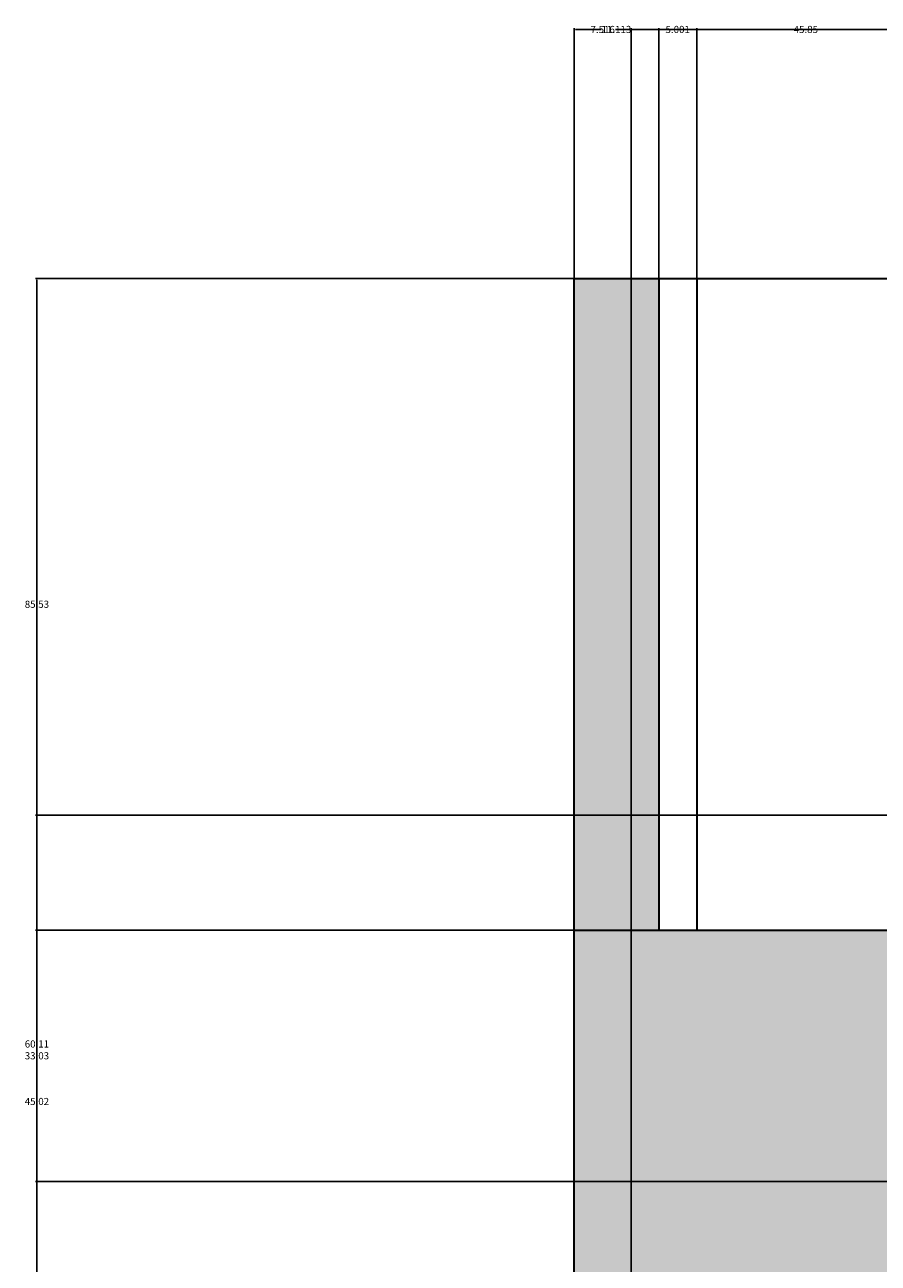
# Model space of a CAD drawing. Units: inches. Extents: x -5 to 714, y 84 to 644.
# Tile 9 of 20: x -4 to 108, y 481 to 644. Entities that reach past the tile are written whole.
import ezdxf

# ---------------------------------------------------------------- set-up
doc = ezdxf.new("R2010")
doc.units = ezdxf.units.IN
doc.header["$MEASUREMENT"] = 0
for name, color, linetype, lineweight in [('A-ANNO-DIMS', 2, 'Continuous', 18), ('A-ELEV', 7, 'Continuous', 35), ('A-ELEV-PATT', 8, 'Continuous', 13)]:
    doc.layers.add(name, color=color, linetype=linetype, lineweight=lineweight)
doc.styles.get("Standard").update_dxf_attribs({"font": 'arial.ttf'})
doc.dimstyles.get("Standard").update_dxf_attribs({"dimtxt": 0.9375, "dimasz": 0.18, "dimexe": 0.18, "dimexo": 0.0625, "dimgap": 0.09, "dimtad": 0, "dimtih": 1, "dimtoh": 1, "dimdec": 4, "dimzin": 0, "dimdsep": 46, "dimlunit": 4, "dimtxsty": 'Standard', "dimcen": 0.09, "dimadec": 0, "dimazin": 0, "dimtfac": 1, "dimtdec": 4, "dimtofl": 0, "dimtmove": 0, "dimatfit": 3, "dimfxl": 1, "dimtolj": 1, "dimtzin": 0, "dimarcsym": 0})

# ---------------------------------------------------------------- blocks, each defined once
blk = doc.blocks.new('*D2')
at = {"layer": 'A-ANNO-DIMS', "color": 0, "lineweight": -2, "transparency": 16777216}
for p, q in [((67.93, 610.73), (-2.74, 610.73)), ((-2.56, 610.55), (-2.56, 364.53)), ((-2.56, 117.37), (-2.56, 363.39)), ((30.08, 117.19), (-2.74, 117.19))]:
    blk.add_line(p, q, dxfattribs=at)
at = {"layer": 'A-ANNO-DIMS', "color": 0, "transparency": 16777216}
for points in [[(-2.59, 610.55), (-2.53, 610.55), (-2.56, 610.73)], [(-2.59, 117.37), (-2.53, 117.37), (-2.56, 117.19)]]:
    blk.add_solid(points, dxfattribs=at)
at = {"layer": 'Defpoints', "color": 0, "transparency": 16777216}
for p in [(-2.56, 610.73), (67.99, 610.73), (30.14, 117.19)]:
    blk.add_point(p, dxfattribs=at)
at = {"layer": 'A-ANNO-DIMS', "color": 0, "transparency": 16777216, "insert": (-2.56, 363.96), "char_height": 0.938, "attachment_point": 5}
blk.add_mtext('\\A1;493.5', dxfattribs=at)
blk = doc.blocks.new('*D6')
at = {"layer": 'A-ANNO-DIMS', "color": 0, "lineweight": -2, "transparency": 16777216}
for p, q in [((67.93, 525.19), (-2.74, 525.19)), ((-2.56, 525.01), (-2.56, 435.76)), ((-2.56, 345.37), (-2.56, 434.62)), ((67.93, 345.19), (-2.74, 345.19))]:
    blk.add_line(p, q, dxfattribs=at)
at = {"layer": 'A-ANNO-DIMS', "color": 0, "transparency": 16777216}
for points in [[(-2.59, 525.01), (-2.53, 525.01), (-2.56, 525.19)], [(-2.59, 345.37), (-2.53, 345.37), (-2.56, 345.19)]]:
    blk.add_solid(points, dxfattribs=at)
at = {"layer": 'Defpoints', "color": 0, "transparency": 16777216}
for p in [(-2.56, 525.19), (67.99, 525.19), (67.99, 345.19)]:
    blk.add_point(p, dxfattribs=at)
at = {"layer": 'A-ANNO-DIMS', "color": 0, "transparency": 16777216, "insert": (-2.56, 435.19), "char_height": 0.938, "attachment_point": 5}
blk.add_mtext('\\A1;180', dxfattribs=at)
blk = doc.blocks.new('*D7')
at = {"layer": 'A-ANNO-DIMS', "color": 0, "lineweight": -2, "transparency": 16777216}
for p, q in [((67.93, 610.73), (-2.74, 610.73)), ((-2.56, 610.55), (-2.56, 568.53)), ((-2.56, 525.37), (-2.56, 567.39)), ((67.93, 525.19), (-2.74, 525.19))]:
    blk.add_line(p, q, dxfattribs=at)
at = {"layer": 'A-ANNO-DIMS', "color": 0, "transparency": 16777216}
for points in [[(-2.59, 610.55), (-2.53, 610.55), (-2.56, 610.73)], [(-2.59, 525.37), (-2.53, 525.37), (-2.56, 525.19)]]:
    blk.add_solid(points, dxfattribs=at)
at = {"layer": 'Defpoints', "color": 0, "transparency": 16777216}
for p in [(-2.56, 610.73), (67.99, 610.73), (67.99, 525.19)]:
    blk.add_point(p, dxfattribs=at)
at = {"layer": 'A-ANNO-DIMS', "color": 0, "transparency": 16777216, "insert": (-2.56, 567.96), "char_height": 0.938, "attachment_point": 5}
blk.add_mtext('\\A1;85.53', dxfattribs=at)
blk = doc.blocks.new('*D8')
at = {"layer": 'A-ANNO-DIMS', "color": 0, "lineweight": -2, "transparency": 16777216}
for p, q in [((67.99, 610.79), (67.99, 643.61)), ((68.17, 643.43), (71.55, 643.43)), ((78.92, 643.43), (75.54, 643.43)), ((79.1, 610.79), (79.1, 643.61))]:
    blk.add_line(p, q, dxfattribs=at)
at = {"layer": 'A-ANNO-DIMS', "color": 0, "transparency": 16777216}
for points in [[(68.17, 643.46), (68.17, 643.4), (67.99, 643.43)], [(78.92, 643.46), (78.92, 643.4), (79.1, 643.43)]]:
    blk.add_solid(points, dxfattribs=at)
at = {"layer": 'Defpoints', "color": 0, "transparency": 16777216}
for p in [(79.1, 643.43), (67.99, 610.73), (79.1, 610.73)]:
    blk.add_point(p, dxfattribs=at)
at = {"layer": 'A-ANNO-DIMS', "color": 0, "transparency": 16777216, "insert": (73.55, 643.43), "char_height": 0.938, "attachment_point": 5}
blk.add_mtext('\\A1;11.113', dxfattribs=at)
blk = doc.blocks.new('*D9')
at = {"layer": 'A-ANNO-DIMS', "color": 0, "lineweight": -2, "transparency": 16777216}
for p, q in [((79.1, 610.79), (79.1, 643.61)), ((79.28, 643.43), (80.02, 643.43)), ((83.92, 643.43), (83.18, 643.43)), ((84.1, 610.79), (84.1, 643.61))]:
    blk.add_line(p, q, dxfattribs=at)
at = {"layer": 'A-ANNO-DIMS', "color": 0, "transparency": 16777216}
for points in [[(79.28, 643.46), (79.28, 643.4), (79.1, 643.43)], [(83.92, 643.46), (83.92, 643.4), (84.1, 643.43)]]:
    blk.add_solid(points, dxfattribs=at)
at = {"layer": 'Defpoints', "color": 0, "transparency": 16777216}
for p in [(84.1, 643.43), (79.1, 610.73), (84.1, 610.73)]:
    blk.add_point(p, dxfattribs=at)
at = {"layer": 'A-ANNO-DIMS', "color": 0, "transparency": 16777216, "insert": (81.6, 643.43), "char_height": 0.938, "attachment_point": 5}
blk.add_mtext('\\A1;5.001', dxfattribs=at)
blk = doc.blocks.new('*D10')
at = {"layer": 'A-ANNO-DIMS', "color": 0, "lineweight": -2, "transparency": 16777216}
for p, q in [((84.1, 610.79), (84.1, 643.61)), ((84.28, 643.43), (139.22, 643.43)), ((198.15, 643.43), (143.21, 643.43)), ((198.33, 610.79), (198.33, 643.61))]:
    blk.add_line(p, q, dxfattribs=at)
at = {"layer": 'A-ANNO-DIMS', "color": 0, "transparency": 16777216}
for points in [[(84.28, 643.46), (84.28, 643.4), (84.1, 643.43)], [(198.15, 643.46), (198.15, 643.4), (198.33, 643.43)]]:
    blk.add_solid(points, dxfattribs=at)
at = {"layer": 'Defpoints', "color": 0, "transparency": 16777216}
for p in [(198.33, 643.43), (84.1, 610.73), (198.33, 610.73)]:
    blk.add_point(p, dxfattribs=at)
at = {"layer": 'A-ANNO-DIMS', "color": 0, "transparency": 16777216, "insert": (141.22, 643.43), "char_height": 0.938, "attachment_point": 5}
blk.add_mtext('\\A1;114.23', dxfattribs=at)
blk = doc.blocks.new('*D16')
at = {"layer": 'A-ANNO-DIMS', "color": 0, "lineweight": -2, "transparency": 16777216}
for p, q in [((364.22, 540.29), (-2.74, 540.29)), ((-2.56, 540.11), (-2.56, 510.8)), ((-2.56, 480.35), (-2.56, 509.66)), ((364.22, 480.17), (-2.74, 480.17))]:
    blk.add_line(p, q, dxfattribs=at)
at = {"layer": 'A-ANNO-DIMS', "color": 0, "transparency": 16777216}
for points in [[(-2.59, 540.11), (-2.53, 540.11), (-2.56, 540.29)], [(-2.59, 480.35), (-2.53, 480.35), (-2.56, 480.17)]]:
    blk.add_solid(points, dxfattribs=at)
at = {"layer": 'Defpoints', "color": 0, "transparency": 16777216}
for p in [(-2.56, 540.29), (364.28, 540.29), (364.28, 480.17)]:
    blk.add_point(p, dxfattribs=at)
at = {"layer": 'A-ANNO-DIMS', "color": 0, "transparency": 16777216, "insert": (-2.56, 510.23), "char_height": 0.938, "attachment_point": 5}
blk.add_mtext('\\A1;60.11', dxfattribs=at)
blk = doc.blocks.new('*D17')
at = {"layer": 'A-ANNO-DIMS', "color": 0, "lineweight": -2, "transparency": 16777216}
for p, q in [((338.04, 525.19), (-2.74, 525.19)), ((-2.56, 525.01), (-2.56, 509.25)), ((-2.56, 492.35), (-2.56, 508.11)), ((338.04, 492.17), (-2.74, 492.17))]:
    blk.add_line(p, q, dxfattribs=at)
at = {"layer": 'A-ANNO-DIMS', "color": 0, "transparency": 16777216}
for points in [[(-2.59, 525.01), (-2.53, 525.01), (-2.56, 525.19)], [(-2.59, 492.35), (-2.53, 492.35), (-2.56, 492.17)]]:
    blk.add_solid(points, dxfattribs=at)
at = {"layer": 'Defpoints', "color": 0, "transparency": 16777216}
for p in [(-2.56, 525.19), (338.11, 525.19), (338.11, 492.17)]:
    blk.add_point(p, dxfattribs=at)
at = {"layer": 'A-ANNO-DIMS', "color": 0, "transparency": 16777216, "insert": (-2.56, 508.68), "char_height": 0.938, "attachment_point": 5}
blk.add_mtext('\\A1;33.03', dxfattribs=at)
blk = doc.blocks.new('*D23')
at = {"layer": 'A-ANNO-DIMS', "color": 0, "lineweight": -2, "transparency": 16777216}
for p, q in [((229.3, 525.19), (-2.74, 525.19)), ((-2.56, 525.01), (-2.56, 503.25)), ((-2.56, 480.35), (-2.56, 502.11)), ((229.3, 480.17), (-2.74, 480.17))]:
    blk.add_line(p, q, dxfattribs=at)
at = {"layer": 'A-ANNO-DIMS', "color": 0, "transparency": 16777216}
for points in [[(-2.59, 525.01), (-2.53, 525.01), (-2.56, 525.19)], [(-2.59, 480.35), (-2.53, 480.35), (-2.56, 480.17)]]:
    blk.add_solid(points, dxfattribs=at)
at = {"layer": 'Defpoints', "color": 0, "transparency": 16777216}
for p in [(-2.56, 525.19), (229.36, 525.19), (229.36, 480.17)]:
    blk.add_point(p, dxfattribs=at)
at = {"layer": 'A-ANNO-DIMS', "color": 0, "transparency": 16777216, "insert": (-2.56, 502.68), "char_height": 0.938, "attachment_point": 5}
blk.add_mtext('\\A1;45.02', dxfattribs=at)
blk = doc.blocks.new('*D46')
at = {"layer": 'A-ANNO-DIMS', "color": 0, "lineweight": -2, "transparency": 16777216}
for p, q in [((67.99, 345.26), (67.99, 643.61)), ((68.17, 643.43), (70.08, 643.43)), ((75.32, 643.43), (73.41, 643.43)), ((75.5, 336.27), (75.5, 643.61))]:
    blk.add_line(p, q, dxfattribs=at)
at = {"layer": 'A-ANNO-DIMS', "color": 0, "transparency": 16777216}
for points in [[(68.17, 643.46), (68.17, 643.4), (67.99, 643.43)], [(75.32, 643.46), (75.32, 643.4), (75.5, 643.43)]]:
    blk.add_solid(points, dxfattribs=at)
at = {"layer": 'Defpoints', "color": 0, "transparency": 16777216}
for p in [(75.5, 643.43), (67.99, 345.19), (75.5, 336.21)]:
    blk.add_point(p, dxfattribs=at)
at = {"layer": 'A-ANNO-DIMS', "color": 0, "transparency": 16777216, "insert": (71.75, 643.43), "char_height": 0.938, "attachment_point": 5}
blk.add_mtext('\\A1;7.516', dxfattribs=at)
blk = doc.blocks.new('*D47')
at = {"layer": 'A-ANNO-DIMS', "color": 0, "lineweight": -2, "transparency": 16777216}
for p, q in [((75.5, 336.27), (75.5, 643.61)), ((75.68, 643.43), (96.74, 643.43)), ((121.18, 643.43), (100.13, 643.43)), ((121.36, 336.27), (121.36, 643.61))]:
    blk.add_line(p, q, dxfattribs=at)
at = {"layer": 'A-ANNO-DIMS', "color": 0, "transparency": 16777216}
for points in [[(75.68, 643.46), (75.68, 643.4), (75.5, 643.43)], [(121.18, 643.46), (121.18, 643.4), (121.36, 643.43)]]:
    blk.add_solid(points, dxfattribs=at)
at = {"layer": 'Defpoints', "color": 0, "transparency": 16777216}
for p in [(121.36, 643.43), (75.5, 336.21), (121.36, 336.21)]:
    blk.add_point(p, dxfattribs=at)
at = {"layer": 'A-ANNO-DIMS', "color": 0, "transparency": 16777216, "insert": (98.43, 643.43), "char_height": 0.938, "attachment_point": 5}
blk.add_mtext('\\A1;45.85', dxfattribs=at)

msp = doc.modelspace()

# ---------------------------------------------------------------- hatches: boundary and pattern name
at = {"layer": 'A-ELEV-PATT', "transparency": 33554687}
h = msp.add_hatch(color=256, dxfattribs=at)
h.dxf.hatch_style = 1
h.paths.add_polyline_path([(79.1019, 610.7276), (67.9893, 610.7276), (67.9893, 525.1928), (79.1019, 525.1928)])
h = msp.add_hatch(color=256, dxfattribs=at)
h.dxf.hatch_style = 1
h.paths.add_polyline_path([(188.3677, 525.1928), (67.9893, 525.1928), (67.9893, 489.1928), (67.9893, 345.1928), (126.7303, 345.1928), (126.7303, 480.1709), (229.3575, 480.1709), (229.3575, 525.1928), (212.6043, 525.1928), (212.6043, 482.7164), (211.0019, 482.7164), (211.0019, 525.1928), (207.6919, 525.1928), (199.9852, 525.1928), (199.9852, 482.7164), (198.3828, 482.7164), (198.3828, 525.1928), (189.9701, 525.1928), (189.9701, 482.7164), (188.3677, 482.7164)])
h.paths.add_polyline_path([(121.3589, 336.2066), (75.5048, 336.2066), (75.5048, 319.345), (121.3589, 319.345)])
h.paths.add_polyline_path([(121.3589, 319.345), (75.5048, 319.345), (75.5048, 302.3045), (121.3589, 302.3045)])
h.paths.add_polyline_path([(121.3589, 302.3045), (75.5048, 302.3045), (75.5048, 282.8561), (121.3589, 282.8561)])
h.paths.add_polyline_path([(121.3589, 282.8561), (75.5048, 282.8561), (75.5048, 261.5556), (121.3589, 261.5556)])
h.paths.add_polyline_path([(121.3589, 261.5556), (75.5048, 261.5556), (75.5048, 243.7009), (121.3589, 243.7009)])
h.paths.add_polyline_path([(121.3589, 243.7009), (75.5048, 243.7009), (75.5048, 223.5117), (121.3589, 223.5117)])
h.paths.add_polyline_path([(121.3589, 223.5117), (75.5048, 223.5117), (75.5048, 212.5836), (121.3589, 212.5836)])
h.paths.add_polyline_path([(121.3589, 212.5836), (75.5048, 212.5836), (75.5048, 201.1928), (121.3589, 201.1928)])
h.paths.add_polyline_path([(179.9335, 201.1928), (30.1395, 201.1928), (30.1395, 198.7054), (179.9335, 198.7054)])
h.paths.add_polyline_path([(187.6349, 201.1928), (179.9335, 201.1928), (179.9335, 198.7054), (179.9335, 141.1928), (269.2446, 141.1928), (269.2446, 201.1928), (263.4349, 201.1928), (263.4349, 152.1176), (187.6349, 152.1176)])
h.paths.add_polyline_path([(269.2446, 277.0513), (269.2446, 287.501), (269.2446, 306.6286), (578.0915, 306.6286), (578.0915, 201.1928), (593.428, 201.1928), (593.428, 315.0968), (584.4202, 315.0968), (259.0665, 315.0968), (259.0665, 201.1928), (263.4349, 201.1928), (269.2446, 201.1928)])

# ---------------------------------------------------------------- linework, layer by layer
at = {"layer": 'A-ELEV'}
for p, q in [((67.9893, 525.1928), (67.9893, 610.7276)), ((67.9893, 610.7276), (79.1019, 610.7276)), ((79.1019, 610.7276), (79.1019, 525.1928)), ((79.1019, 610.7276), (198.3291, 610.7276)), ((84.1027, 610.7276), (84.1027, 525.1928)), ((67.9893, 489.1928), (67.9893, 525.1928)), ((67.9893, 525.1928), (207.6919, 525.1928)), ((67.9893, 345.1928), (67.9893, 489.1928))]:
    msp.add_line(p, q, dxfattribs=at)

# ---------------------------------------------------------------- dimensions: what is measured, and where the dimension line sits
at = {"layer": 'A-ANNO-DIMS'}
for base, p1, p2, override, picture, middle in [((79.1019, 643.4276), (67.9893, 610.7276), (79.1019, 610.7276), {"dimdec": 3, "dimlfac": 1, "dimrnd": 0, "dimzin": 0, "dimdsep": 46, "dimlunit": 2}, '*D8', (73.5456, 643.4276)), ((75.50483, 643.42757), (67.9893, 345.19283), (75.50483, 336.20661), {"dimdec": 3, "dimlfac": 1, "dimrnd": 0, "dimzin": 0, "dimdsep": 46, "dimlunit": 2}, '*D46', (71.74706, 643.42757)), ((121.3589, 643.4276), (75.5048, 336.2066), (121.3589, 336.2066), {"dimdec": 2, "dimlfac": 1, "dimrnd": 0, "dimzin": 0, "dimdsep": 46, "dimlunit": 2}, '*D47', (98.4319, 643.4276)), ((84.1027, 643.4276), (79.1019, 610.7276), (84.1027, 610.7276), {"dimdec": 3, "dimlfac": 1, "dimrnd": 0, "dimzin": 0, "dimdsep": 46, "dimlunit": 2}, '*D9', (81.6023, 643.4276)), ((198.3291, 643.4276), (84.1027, 610.7276), (198.3291, 610.7276), {"dimdec": 2, "dimlfac": 1, "dimrnd": 0, "dimzin": 0, "dimdsep": 46, "dimlunit": 2}, '*D10', (141.2159, 643.4276))]:
    dim = msp.add_linear_dim(base=base, p1=p1, p2=p2, dimstyle='Standard', override=override, dxfattribs=at)
    dim.commit()
    dim.dimension.update_dxf_attribs({"geometry": picture, "text_midpoint": middle})
for base, p1, p2, override, picture, middle in [((-2.5605, 610.7276), (30.1395, 117.1928), (67.9893, 610.7276), {"dimdec": 1, "dimlfac": 1, "dimrnd": 0, "dimzin": 0, "dimdsep": 46, "dimlunit": 2}, '*D2', (-2.5605, 363.9602)), ((-2.5605, 610.7276), (67.9893, 525.1928), (67.9893, 610.7276), {"dimdec": 2, "dimlfac": 1, "dimrnd": 0, "dimzin": 0, "dimdsep": 46, "dimlunit": 2}, '*D7', (-2.5605, 567.9602)), ((-2.5605, 540.2857), (364.2809, 480.1709), (364.2809, 540.2857), {"dimdec": 2, "dimlfac": 1, "dimrnd": 0, "dimzin": 0, "dimdsep": 46, "dimlunit": 2}, '*D16', (-2.5605, 510.2283)), ((-2.5605, 525.1928), (338.106, 492.1651), (338.106, 525.1928), {"dimdec": 2, "dimlfac": 1, "dimrnd": 0, "dimzin": 0, "dimdsep": 46, "dimlunit": 2}, '*D17', (-2.5605, 508.679)), ((-2.5605, 525.1928), (229.3575, 480.1709), (229.3575, 525.1928), {"dimdec": 2, "dimlfac": 1, "dimrnd": 0, "dimzin": 0, "dimdsep": 46, "dimlunit": 2}, '*D23', (-2.5605, 502.6819)), ((-2.5605, 525.1928), (67.9893, 345.1928), (67.9893, 525.1928), {"dimdec": 0, "dimlfac": 1, "dimrnd": 0, "dimzin": 0, "dimdsep": 46, "dimlunit": 2}, '*D6', (-2.5605, 435.1928))]:
    dim = msp.add_linear_dim(base=base, p1=p1, p2=p2, angle=90, dimstyle='Standard', override=override, dxfattribs=at)
    dim.commit()
    dim.dimension.update_dxf_attribs({"geometry": picture, "text_midpoint": middle})

doc.saveas('drawing.dxf')
